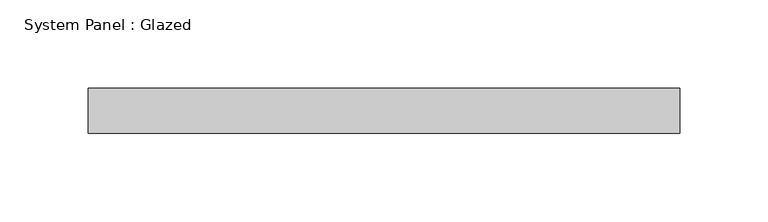
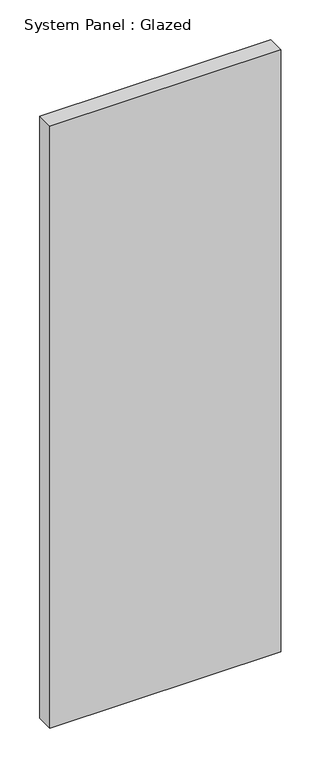
"""IFC4 building model written with IfcOpenShell, lengths in millimetres: plate geometry, System Panel : Glazed."""

from ifc_helpers import new_model, si_unit, origin, origin_with_axes, place, context, project, spatial, polyline, outline, extrude, source, transform, mapped, element, save


def system_panel_glazed_299ce7ab(model_context):
    return source(origin(), model_context, "Body", "SweptSolid", [
        extrude(outline(polyline([(167.4822706, 19.05), (-167.4822706, 19.05), (-167.4822706, 44.45), (167.4822706, 44.45), (167.4822706, 19.05)])), origin_with_axes(), (0.0, 0.0, 1.0), 923.1640555),
    ])


if __name__ == "__main__":
    model = new_model("IFC4")
    model_context = context("Model", 3, world=origin())
    ifc_project = project(units=[si_unit("LENGTHUNIT", "METRE", prefix="MILLI")], contexts=[model_context])
    site = spatial("IfcSite", under=ifc_project)
    building = spatial("IfcBuilding", under=site)
    placement = place(None, origin())
    system_panel_glazed_shape = system_panel_glazed_299ce7ab(model_context)
    element("IfcPlate", 1, ObjectType="System Panel : Glazed", at=placement, inside=building, context=model_context, shape_type="MappedRepresentation", body=[
        mapped(system_panel_glazed_shape, transform((0.0, 0.0, 0.0), x_axis=(1.0, 0.0, 0.0), y_axis=(0.0, 1.0, 0.0), z_axis=(0.0, 0.0, 1.0))),
    ])
    save(model, "model.ifc")

# Revit data of these elements
# Type "System Panel : Glazed"
#   Construction Type Id = "GSP4R"
#   Analytic Construction = "1/8 in Pilkington single glazing"
#   Visual Light Transmittance = 0.9
#   Solar Heat Gain Coefficient = 0.86
#   Heat Transfer Coefficient (U) = 1.18115 BTU/(h·ft²·°F)
# Element 1 (IfcPlate, "System Panel : Glazed")
#   Materials on its faces: "Glass"
# Materials
#   "Glass": class "Glass", colour RGB 0 128 192, transparency 0.75, Description = "Soda Lime Glass", Cost = 0
